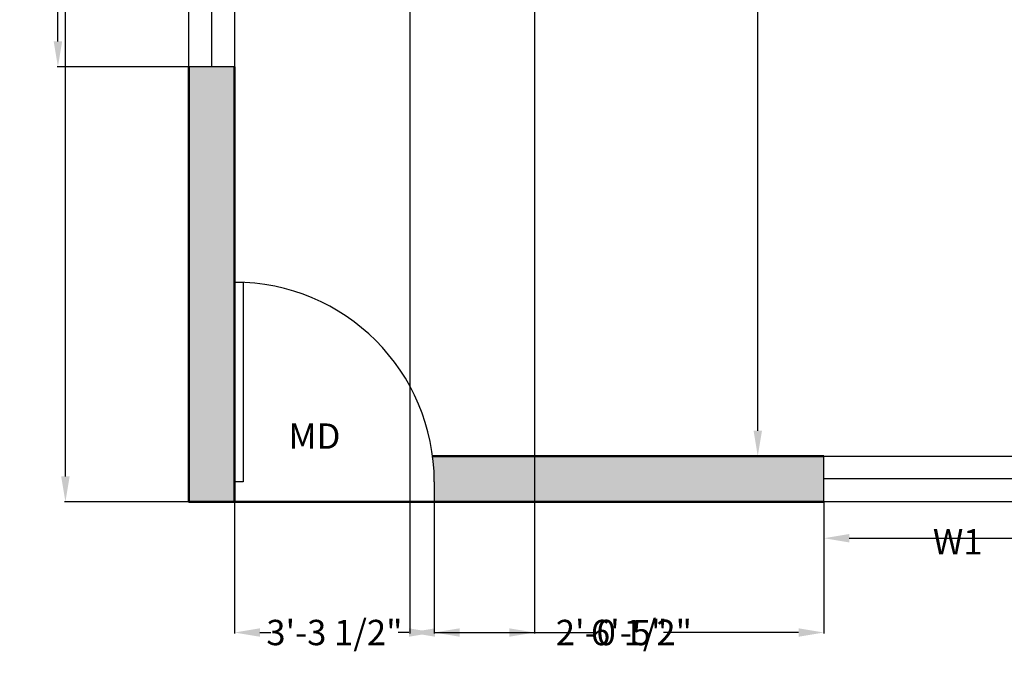
# Model space of a CAD drawing. Units: inches. Extents: x 3136 to 3620, y 13606 to 14152.
# Tile 1 of 6: x 3192 to 3386, y 13606 to 13734. Entities that reach past the tile are written whole.
import ezdxf

# ---------------------------------------------------------------- set-up
doc = ezdxf.new("R2010")
doc.units = ezdxf.units.IN
for name, color, linetype, lineweight in [('A-ANNO-DIMS', 2, 'Continuous', 18), ('A-ANNO-TEXT', 7, 'Continuous', 18), ('A-DOOR', 3, 'Continuous', 25), ('A-GLAZ', 4, 'Continuous', 25), ('A-WALL', 7, 'Continuous', 50), ('A-WALL-PATT', 174, 'Continuous', 13)]:
    doc.layers.add(name, color=color, linetype=linetype, lineweight=lineweight)
doc.styles.get("Standard").update_dxf_attribs({"font": 'arial.ttf', "height": 5})
doc.dimstyles.get("Standard").update_dxf_attribs({"dimtxt": 5, "dimasz": 5, "dimexe": 0.18, "dimexo": 0.0625, "dimgap": 0.09, "dimtad": 0, "dimtih": 1, "dimtoh": 1, "dimdec": 0, "dimzin": 0, "dimdsep": 46, "dimlunit": 3, "dimtxsty": 'Standard', "dimcen": 0.09, "dimadec": 0, "dimazin": 0, "dimtfac": 1, "dimtdec": 0, "dimtofl": 0, "dimtmove": 0, "dimatfit": 3, "dimfxl": 1, "dimtolj": 1, "dimtzin": 0, "dimarcsym": 0})

# ---------------------------------------------------------------- blocks, each defined once
blk = doc.blocks.new('*U2')
for p, q in [((0, 0), (0, -100)), ((1000, 0), (1000, -100))]:
    blk.add_line(p, q)
blk.add_lwpolyline([(0, 0), (0, 1000), (43.75, 1000), (43.75, 0)], close=True)
blk.add_arc((0, 0), 1000, 0, 90)
blk = doc.blocks.new('*D16')
at = {"layer": 'A-ANNO-DIMS', "color": 0, "lineweight": -2, "transparency": 16777216}
for p, q in [((3311.54, 13851.84), (3337.17, 13851.84)), ((3336.99, 13846.84), (3336.99, 13752.44)), ((3336.99, 13652.84), (3336.99, 13747.24)), ((3311.54, 13647.84), (3337.17, 13647.84))]:
    blk.add_line(p, q, dxfattribs=at)
at = {"layer": 'A-ANNO-DIMS', "color": 0, "transparency": 16777216}
for points in [[(3336.16, 13846.84), (3337.82, 13846.84), (3336.99, 13851.84)], [(3336.16, 13652.84), (3337.82, 13652.84), (3336.99, 13647.84)]]:
    blk.add_solid(points, dxfattribs=at)
at = {"layer": 'Defpoints', "color": 0, "transparency": 16777216}
for p in [(3311.47, 13851.84), (3336.99, 13851.84), (3311.47, 13647.84)]:
    blk.add_point(p, dxfattribs=at)
at = {"layer": 'A-ANNO-DIMS', "color": 0, "transparency": 16777216, "insert": (3336.99, 13749.84), "char_height": 5, "attachment_point": 5}
blk.add_mtext("\\A1;17'", dxfattribs=at)
blk = doc.blocks.new('*D28')
at = {"layer": 'A-ANNO-DIMS', "color": 0, "lineweight": -2, "transparency": 16777216}
for p, q in [((3224.81, 14118.84), (3200.37, 14118.84)), ((3200.55, 14113.84), (3200.55, 13881.48)), ((3200.55, 13643.84), (3200.55, 13876.2)), ((3224.81, 13638.84), (3200.37, 13638.84))]:
    blk.add_line(p, q, dxfattribs=at)
at = {"layer": 'A-ANNO-DIMS', "color": 0, "transparency": 16777216}
for points in [[(3199.71, 14113.84), (3201.38, 14113.84), (3200.55, 14118.84)], [(3199.71, 13643.84), (3201.38, 13643.84), (3200.55, 13638.84)]]:
    blk.add_solid(points, dxfattribs=at)
at = {"layer": 'Defpoints', "color": 0, "transparency": 16777216}
for p in [(3200.55, 14118.84), (3224.87, 14118.84), (3224.87, 13638.84)]:
    blk.add_point(p, dxfattribs=at)
at = {"layer": 'A-ANNO-DIMS', "color": 0, "transparency": 16777216, "insert": (3200.55, 13878.84), "char_height": 5, "attachment_point": 5}
blk.add_mtext("\\A1;40'", dxfattribs=at)
blk = doc.blocks.new('WIN-48IN-GLAZING')
for p, q in [((0, 0), (0, 9)), ((48, 0), (48, 9)), ((48, 4.5), (0, 4.5))]:
    blk.add_line(p, q)
blk = doc.blocks.new('*D30')
at = {"layer": 'A-ANNO-DIMS', "color": 0, "lineweight": -2, "transparency": 16777216}
for p, q in [((3350.03, 13638.78), (3350.03, 13631.46)), ((3398.03, 13638.78), (3398.03, 13631.46)), ((3355.03, 13631.64), (3393.03, 13631.64)), ((3398.03, 13631.64), (3403.03, 13631.64))]:
    blk.add_line(p, q, dxfattribs=at)
at = {"layer": 'A-ANNO-DIMS', "color": 0, "transparency": 16777216}
for points in [[(3355.03, 13632.47), (3355.03, 13630.81), (3350.03, 13631.64)], [(3393.03, 13632.47), (3393.03, 13630.81), (3398.03, 13631.64)]]:
    blk.add_solid(points, dxfattribs=at)
at = {"layer": 'Defpoints', "color": 0, "transparency": 16777216}
for p in [(3350.03, 13638.84), (3398.03, 13638.84), (3398.03, 13631.64)]:
    blk.add_point(p, dxfattribs=at)
at = {"layer": 'A-ANNO-DIMS', "color": 0, "transparency": 16777216, "insert": (3434.76, 13631.64), "char_height": 5, "attachment_point": 5}
blk.add_mtext('\\A1;WINDOW 4\'-0" TYP.', dxfattribs=at)
blk = doc.blocks.new('*D46')
at = {"layer": 'A-ANNO-DIMS', "color": 0, "lineweight": -2, "transparency": 16777216}
for p, q in [((3233.87, 13638.78), (3233.87, 13612.86)), ((3273.24, 13638.78), (3273.24, 13612.86)), ((3238.87, 13613.04), (3241, 13613.04)), ((3268.24, 13613.04), (3266.12, 13613.04))]:
    blk.add_line(p, q, dxfattribs=at)
at = {"layer": 'A-ANNO-DIMS', "color": 0, "transparency": 16777216}
for points in [[(3238.87, 13613.87), (3238.87, 13612.21), (3233.87, 13613.04)], [(3268.24, 13613.87), (3268.24, 13612.21), (3273.24, 13613.04)]]:
    blk.add_solid(points, dxfattribs=at)
at = {"layer": 'Defpoints', "color": 0, "transparency": 16777216}
for p in [(3233.87, 13638.84), (3273.24, 13638.84), (3273.24, 13613.04)]:
    blk.add_point(p, dxfattribs=at)
at = {"layer": 'A-ANNO-DIMS', "color": 0, "transparency": 16777216, "insert": (3253.56, 13613.04), "char_height": 5, "attachment_point": 5}
blk.add_mtext('\\A1;3\'-3 1/2"', dxfattribs=at)
blk = doc.blocks.new('*D51')
at = {"layer": 'A-ANNO-DIMS', "color": 0, "lineweight": -2, "transparency": 16777216}
for p, q in [((3224.81, 13760.63), (3198.89, 13760.63)), ((3199.07, 13755.63), (3199.07, 13745.27)), ((3199.07, 13729.63), (3199.07, 13739.99)), ((3224.81, 13724.63), (3198.89, 13724.63))]:
    blk.add_line(p, q, dxfattribs=at)
at = {"layer": 'A-ANNO-DIMS', "color": 0, "transparency": 16777216}
for points in [[(3198.24, 13755.63), (3199.9, 13755.63), (3199.07, 13760.63)], [(3198.24, 13729.63), (3199.9, 13729.63), (3199.07, 13724.63)]]:
    blk.add_solid(points, dxfattribs=at)
at = {"layer": 'Defpoints', "color": 0, "transparency": 16777216}
for p in [(3199.07, 13760.63), (3224.87, 13760.63), (3224.87, 13724.63)]:
    blk.add_point(p, dxfattribs=at)
at = {"layer": 'A-ANNO-DIMS', "color": 0, "transparency": 16777216, "insert": (3199.07, 13742.63), "char_height": 5, "attachment_point": 5}
blk.add_mtext('\\A1;3\'-0"', dxfattribs=at)
blk = doc.blocks.new('*D57')
at = {"layer": 'A-ANNO-DIMS', "color": 0, "lineweight": -2, "transparency": 16777216}
for p, q in [((3273.24, 13638.78), (3273.24, 13612.86)), ((3350.03, 13638.78), (3350.03, 13612.86)), ((3278.24, 13613.04), (3304.89, 13613.04)), ((3345.03, 13613.04), (3318.39, 13613.04))]:
    blk.add_line(p, q, dxfattribs=at)
at = {"layer": 'A-ANNO-DIMS', "color": 0, "transparency": 16777216}
for points in [[(3278.24, 13613.87), (3278.24, 13612.21), (3273.24, 13613.04)], [(3345.03, 13613.87), (3345.03, 13612.21), (3350.03, 13613.04)]]:
    blk.add_solid(points, dxfattribs=at)
at = {"layer": 'Defpoints', "color": 0, "transparency": 16777216}
for p in [(3273.24, 13638.84), (3350.03, 13638.84), (3350.03, 13613.04)]:
    blk.add_point(p, dxfattribs=at)
at = {"layer": 'A-ANNO-DIMS', "color": 0, "transparency": 16777216, "insert": (3311.64, 13613.04), "char_height": 5, "attachment_point": 5}
blk.add_mtext('\\A1;6\'-5"', dxfattribs=at)
blk = doc.blocks.new('*D76')
at = {"layer": 'A-ANNO-DIMS', "color": 0, "lineweight": -2, "transparency": 16777216}
for p, q in [((3293.01, 13742.77), (3293.01, 13612.86)), ((3268.4, 13737.45), (3268.4, 13612.86)), ((3273.4, 13613.04), (3288.01, 13613.04)), ((3293.01, 13613.04), (3298.01, 13613.04))]:
    blk.add_line(p, q, dxfattribs=at)
at = {"layer": 'A-ANNO-DIMS', "color": 0, "transparency": 16777216}
for points in [[(3273.4, 13613.87), (3273.4, 13612.21), (3268.4, 13613.04)], [(3288.01, 13613.87), (3288.01, 13612.21), (3293.01, 13613.04)]]:
    blk.add_solid(points, dxfattribs=at)
at = {"layer": 'Defpoints', "color": 0, "transparency": 16777216}
for p in [(3293.01, 13742.83), (3268.4, 13737.52), (3293.01, 13613.04)]:
    blk.add_point(p, dxfattribs=at)
at = {"layer": 'A-ANNO-DIMS', "color": 0, "transparency": 16777216, "insert": (3310.61, 13613.04), "char_height": 5, "attachment_point": 5}
blk.add_mtext('\\A1;2\'-0 1/2"', dxfattribs=at)

msp = doc.modelspace()

# ---------------------------------------------------------------- hatches: boundary and pattern name
at = {"layer": 'A-WALL-PATT'}
h = msp.add_hatch(color=256, dxfattribs=at)
h.dxf.hatch_style = 1
h.paths.add_polyline_path([(3584.87, 13767.84), (3575.87, 13767.84), (3575.87, 13714.7), (3584.87, 13714.7)])
h.paths.add_polyline_path([(3584.87, 13666.7), (3575.87, 13666.7), (3575.87, 13647.84), (3398.03, 13647.84), (3398.03, 13638.84), (3584.87, 13638.84)])
h.paths.add_polyline_path([(3350.03, 13647.84), (3272.91, 13647.84, -0.03225), (3273.24, 13642.78), (3273.24, 13638.84), (3350.03, 13638.84)])
h.paths.add_polyline_path([(3233.87, 13724.63), (3224.87, 13724.63), (3224.87, 13638.84), (3233.87, 13638.84), (3233.87, 13642.78), (3233.87, 13682.15)])
h.paths.add_polyline_path([(3233.87, 13893.84), (3224.87, 13893.84), (3224.87, 13760.63), (3233.87, 13760.63)])
h.paths.add_polyline_path([(3356.82, 13857.84), (3233.87, 13857.84), (3233.87, 13851.84), (3356.82, 13851.84)])
h.paths.add_polyline_path([(3233.87, 14022.84), (3224.87, 14022.84), (3224.87, 13941.84), (3233.87, 13941.84)])
h.paths.add_polyline_path([(3311.51, 13983.84), (3233.87, 13983.84), (3233.87, 13977.84), (3311.51, 13977.84)])
h.paths.add_polyline_path([(3467.87, 14118.84), (3224.87, 14118.84), (3224.87, 14070.84), (3233.87, 14070.84), (3233.87, 14081.66), (3233.87, 14109.84), (3467.87, 14109.84)])
h.paths.add_polyline_path([(3575.87, 13935.84), (3435.35, 13935.84, -0.018734), (3435.43, 13933.78), (3435.43, 13929.84), (3575.87, 13929.84)])
h.paths.add_polyline_path([(3417.35, 13932.93), (3424.89, 13932.93), (3424.89, 13943.24), (3417.35, 13943.24)], flags=9)
h.paths.add_polyline_path([(3561.82, 13786.65), (3573.42, 13786.65), (3573.42, 13796.96), (3561.82, 13796.96)], flags=9)
h.paths.add_polyline_path([(3567.12, 13888.65), (3574.84, 13888.65), (3574.84, 13898.96), (3567.12, 13898.96)], flags=9)
h.paths.add_polyline_path([(3536.01, 13916.38), (3543.73, 13916.38), (3543.73, 13926.69), (3536.01, 13926.69)], flags=9)
h.paths.add_polyline_path([(3509.85, 13733.24), (3521.46, 13733.24), (3521.46, 13743.54), (3509.85, 13743.54)], flags=9)
h.paths.add_polyline_path([(3499.97, 13866.95), (3511.39, 13866.95), (3511.39, 13877.25), (3499.97, 13877.25)], flags=9)
h.paths.add_polyline_path([(3456.03, 13744.65), (3463.57, 13744.65), (3463.57, 13754.96), (3456.03, 13754.96)], flags=9)

# ---------------------------------------------------------------- linework, layer by layer
at = {"layer": 'A-GLAZ'}
for p, q in [((3229.37, 13724.63), (3229.37, 13760.63)), ((3233.87, 13724.63), (3224.87, 13724.63))]:
    msp.add_line(p, q, dxfattribs=at)
for points in [[(3224.87, 13760.63), (3233.87, 13760.63), (3233.87, 13724.63), (3224.87, 13724.63)], [(3350.03, 13647.84), (3398.03, 13647.84), (3398.03, 13638.84), (3350.03, 13638.84)]]:
    msp.add_lwpolyline(points, close=True, dxfattribs=at)
at = {"layer": 'A-WALL'}
for p, q in [((3233.87, 13647.84), (3233.87, 13724.63)), ((3233.87, 13647.84), (3233.87, 13638.84)), ((3350.03, 13647.84), (3272.91, 13647.84))]:
    msp.add_line(p, q, dxfattribs=at)
msp.add_lwpolyline([(3350.03, 13638.84), (3224.87, 13638.84), (3224.87, 13724.63)], dxfattribs=at)

# ---------------------------------------------------------------- block references
at = {"layer": 'A-DOOR', "xscale": 0.0393700787401575, "yscale": 0.0393700787401575, "zscale": 0.0393700787401575}
msp.add_blockref('*U2', (3233.87, 13642.78), dxfattribs=at)
at = {"layer": 'A-GLAZ'}
msp.add_blockref('WIN-48IN-GLAZING', (3350.03, 13638.84), dxfattribs=at)

# ---------------------------------------------------------------- texts
at = {"layer": 'A-ANNO-TEXT', "char_height": 5, "attachment_point": 1}
for s, width, insert in [('MD', 14.8236, (3244.51, 13654.28)), ('\\pxqc;W1', 22.2613, (3365.26, 13633.43))]:
    msp.add_mtext_dynamic_manual_height_columns(s, width=width, gutter_width=25, heights=[0], dxfattribs=dict(at, insert=insert))

# ---------------------------------------------------------------- dimensions: what is measured, and where the dimension line sits
at = {"layer": 'A-ANNO-DIMS'}
for base, p1, p2, override, picture, middle in [((3200.55, 14118.84), (3224.87, 13638.84), (3224.87, 14118.84), {"dimclrd": 0, "dimclre": 0, "dimclrt": 0}, '*D28', (3200.55, 13878.84)), ((3199.07, 13760.63), (3224.87, 13724.63), (3224.87, 13760.63), {"dimdec": 1, "dimlfac": 1, "dimrnd": 0, "dimzin": 1, "dimdsep": 46, "dimlunit": 4, "dimfrac": 2}, '*D51', (3199.07, 13742.63))]:
    dim = msp.add_linear_dim(base=base, p1=p1, p2=p2, angle=90, dimstyle='Standard', override=override, dxfattribs=at)
    dim.commit()
    dim.dimension.update_dxf_attribs({"geometry": picture, "text_midpoint": middle})
dim = msp.add_linear_dim(base=(3336.99, 13851.84), p1=(3311.47, 13647.84), p2=(3311.47, 13851.84), angle=90, dimstyle='Standard', override={"dimclrd": 0, "dimclre": 0, "dimclrt": 0}, dxfattribs=at)
dim.commit()
dim.dimension.update_dxf_attribs({"geometry": '*D16', "text_midpoint": (3336.99, 13749.84), "dimtype": 160})
for base, p1, p2, picture, middle in [((3293.01, 13613.04), (3268.4, 13737.52), (3293.01, 13742.83), '*D76', (3310.61, 13613.04)), ((3273.24, 13613.04), (3233.87, 13638.84), (3273.24, 13638.84), '*D46', (3253.56, 13613.04)), ((3350.03, 13613.04), (3273.24, 13638.84), (3350.03, 13638.84), '*D57', (3311.64, 13613.04))]:
    dim = msp.add_linear_dim(base=base, p1=p1, p2=p2, dimstyle='Standard', override={"dimdec": 1, "dimlfac": 1, "dimrnd": 0, "dimzin": 1, "dimdsep": 46, "dimlunit": 4, "dimfrac": 2}, dxfattribs=at)
    dim.commit()
    dim.dimension.update_dxf_attribs({"geometry": picture, "text_midpoint": middle})
dim = msp.add_linear_dim(base=(3398.03, 13631.64), p1=(3350.03, 13638.84), p2=(3398.03, 13638.84), text='WINDOW <> TYP.', dimstyle='Standard', override={"dimdec": 1, "dimlfac": 1, "dimrnd": 0, "dimzin": 1, "dimdsep": 46, "dimlunit": 4, "dimfrac": 2}, dxfattribs=at)
dim.commit()
dim.dimension.update_dxf_attribs({"geometry": '*D30', "text_midpoint": (3434.76, 13631.64)})

doc.saveas('drawing.dxf')
